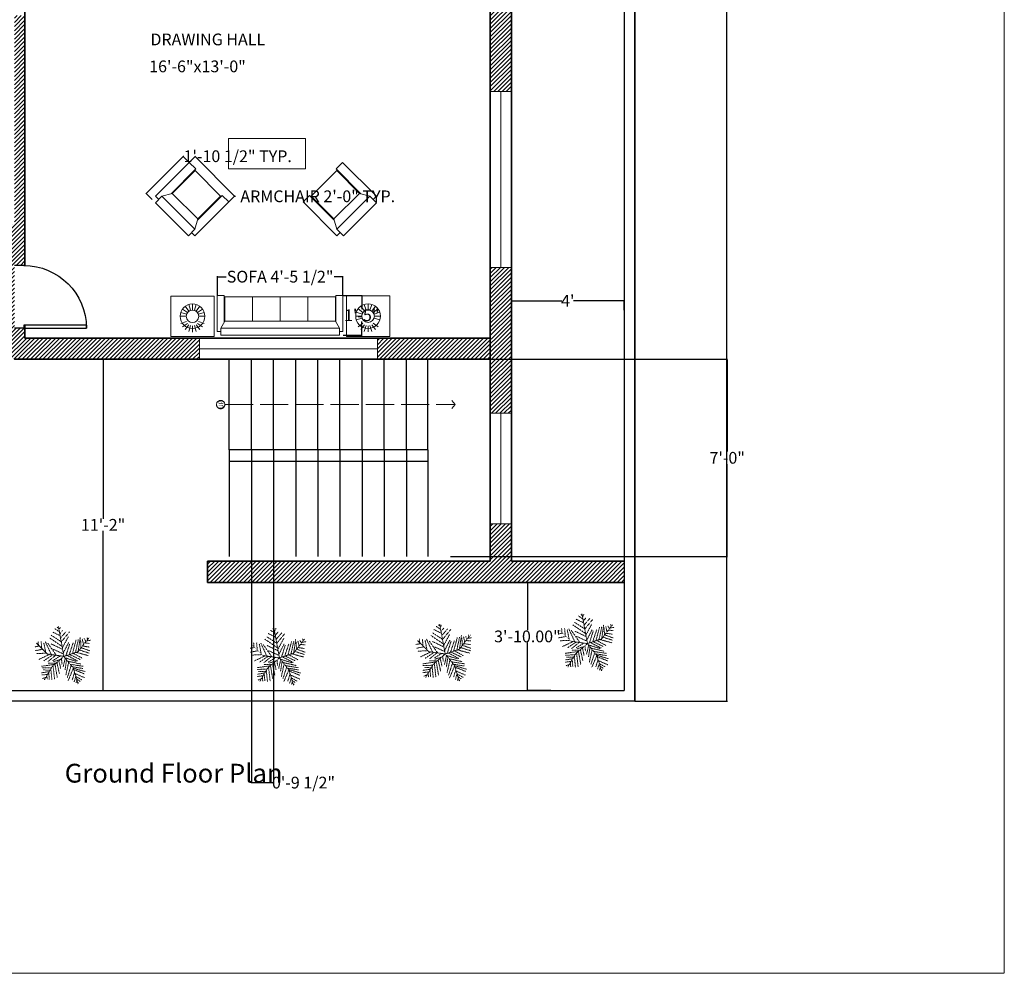
# Model space of a CAD drawing. Units: inches. Extents: x 2202345 to 2203065, y -970921 to -970107.
# Tile 2 of 5: x 2202646 to 2203065, y -970921 to -970515. Entities that reach past the tile are written whole.
import ezdxf

# ---------------------------------------------------------------- set-up
doc = ezdxf.new("R2010")
doc.units = ezdxf.units.IN
doc.header["$MEASUREMENT"] = 0
doc.linetypes.add('ACAD_ISO02W100', pattern=[15, 12, -3])
doc.linetypes.add('HIDDEN', pattern=[0.375, 0.25, -0.125])
doc.layers.get('0').update_dxf_attribs({"color": 13})
for name, color, linetype, lineweight in [('A-ANNO-DIMS', 2, 'Continuous', 18), ('A-ANNO-SYMB', 7, 'ACAD_ISO02W100', 18), ('A-ANNO-TEXT', 7, 'Continuous', 25), ('A-ANNO-TTLB', 7, 'HIDDEN', 18), ('A-AREA-IDEN', 7, 'Continuous', 18), ('A-FLOR-STRS', 252, 'Continuous', 25), ('A-WALL-PATT', 8, 'Continuous', 13), ('C-PROP', 7, 'Continuous', 25), ('doors', 252, 'Continuous', 25), ('furniture', 250, 'Continuous', 18), ('garden', 114, 'HIDDEN', 13), ('walls', 252, 'Continuous', 35), ('windows', 173, 'Continuous', 18)]:
    doc.layers.add(name, color=color, linetype=linetype, lineweight=lineweight)
doc.styles.get("Standard").update_dxf_attribs({"font": 'arial.ttf'})
doc.dimstyles.get("Standard").update_dxf_attribs({"dimtxt": 5, "dimasz": 0.18, "dimexe": 0.18, "dimexo": 0.0625, "dimgap": 0.09, "dimtad": 0, "dimtih": 1, "dimtoh": 1, "dimzin": 0, "dimdsep": 46, "dimlunit": 3, "dimtxsty": 'Standard', "dimcen": 0.09, "dimadec": 0, "dimazin": 0, "dimtfac": 1, "dimtofl": 0, "dimtmove": 0, "dimatfit": 3, "dimfxl": 1, "dimtolj": 1, "dimtzin": 0, "dimarcsym": 0})

# ---------------------------------------------------------------- blocks, each defined once
blk = doc.blocks.new('FABRIC SOFA 4S')
at = {"layer": 'furniture'}
for p, q in [((0, -51), (0, 51)), ((6, 51), (0, 51)), ((3, 54), (34, 54)), ((3, 51), (3, 54)), ((6, -51), (6, 51)), ((12, 47.63), (6, 51)), ((34, 48), (34, 54)), ((11.14, 48), (34, 48)), ((33, 23.81), (12, 23.81)), ((33, 0), (12, 0)), ((33, -23.81), (12, -23.81)), ((6, -51), (12, -47.63)), ((11.54, -48), (34, -48)), ((34, -48), (34, -54)), ((6, -51), (0, -51)), ((3, -54), (3, -51)), ((3, -54), (34, -54))]:
    blk.add_line(p, q, dxfattribs=at)
blk.add_lwpolyline([(12, -47.63), (12, 47.63), (33, 47.63), (33, -47.63)], close=True, dxfattribs=at)
blk = doc.blocks.new('FABRIC SOFA 1S')
at = {"layer": 'furniture'}
for p, q in [((0, -15.12), (0, 15.12)), ((6, 15.12), (0, 15.12)), ((3, 18.12), (34, 18.12)), ((3, 15.12), (3, 18.12)), ((6, -15.12), (6, 15.12)), ((12, 11.75), (6, 15.12)), ((34, 12.12), (34, 18.12)), ((11.33, 12.12), (34, 12.12)), ((6, -15.12), (12, -11.75)), ((11.33, -12.12), (34, -12.12)), ((34, -12.12), (34, -18.12)), ((6, -15.12), (0, -15.12)), ((3, -18.12), (3, -15.12)), ((3, -18.12), (34, -18.12))]:
    blk.add_line(p, q, dxfattribs=at)
blk.add_lwpolyline([(12, -11.75), (12, 11.75), (33, 11.75), (33, -11.75)], close=True, dxfattribs=at)
blk = doc.blocks.new('*U12')
for p, q in [((0, 0), (0, -6)), ((40, 0), (40, -6))]:
    blk.add_line(p, q)
blk.add_lwpolyline([(0, 0), (0, 40), (1.75, 40), (1.75, 0)], close=True)
blk.add_arc((0, 0), 40, 0, 90)
blk = doc.blocks.new('*D17')
at = {"layer": 'A-ANNO-DIMS', "color": 0, "lineweight": -2, "transparency": 16777216}
for p, q in [((2202675.26, -970659.11), (2202681.61, -970659.11)), ((2202681.43, -970659.29), (2202681.43, -970727.01)), ((2202681.43, -970799.93), (2202681.43, -970732.21)), ((2202681.49, -970800.11), (2202681.61, -970800.11))]:
    blk.add_line(p, q, dxfattribs=at)
at = {"layer": 'A-ANNO-DIMS', "color": 0, "transparency": 16777216}
for points in [[(2202681.4, -970659.29), (2202681.46, -970659.29), (2202681.43, -970659.11)], [(2202681.4, -970799.93), (2202681.46, -970799.93), (2202681.43, -970800.11)]]:
    blk.add_solid(points, dxfattribs=at)
at = {"layer": 'Defpoints', "color": 0, "transparency": 16777216}
for p in [(2202675.19, -970659.11), (2202681.43, -970800.11), (2202681.43, -970800.11)]:
    blk.add_point(p, dxfattribs=at)
at = {"layer": 'A-ANNO-DIMS', "color": 0, "transparency": 16777216, "insert": (2202681.43, -970729.61), "char_height": 5, "attachment_point": 5}
blk.add_mtext('\\A1;11\'-2"', dxfattribs=at)
blk = doc.blocks.new('*D18')
at = {"layer": 'A-ANNO-DIMS', "color": 0, "lineweight": -2, "transparency": 16777216}
for p, q in [((2202871.99, -970754.11), (2202861.81, -970754.11)), ((2202861.99, -970754.29), (2202861.99, -970774.46)), ((2202861.99, -970799.93), (2202861.99, -970779.75)), ((2202871.99, -970800.11), (2202861.81, -970800.11))]:
    blk.add_line(p, q, dxfattribs=at)
at = {"layer": 'A-ANNO-DIMS', "color": 0, "transparency": 16777216}
for points in [[(2202861.96, -970754.29), (2202862.02, -970754.29), (2202861.99, -970754.11)], [(2202861.96, -970799.93), (2202862.02, -970799.93), (2202861.99, -970800.11)]]:
    blk.add_solid(points, dxfattribs=at)
at = {"layer": 'Defpoints', "color": 0, "transparency": 16777216}
for p in [(2202872.05, -970754.11), (2202861.99, -970800.11), (2202872.05, -970800.11)]:
    blk.add_point(p, dxfattribs=at)
at = {"layer": 'A-ANNO-DIMS', "color": 0, "transparency": 16777216, "insert": (2202861.99, -970777.11), "char_height": 5, "attachment_point": 5}
blk.add_mtext('\\A1;3\'-10.00"', dxfattribs=at)
blk = doc.blocks.new('*D19')
at = {"layer": 'A-ANNO-DIMS', "color": 0, "lineweight": -2, "transparency": 16777216}
for p, q in [((2202855.18, -970638.23), (2202855.18, -970634)), ((2202855.36, -970634.18), (2202876.69, -970634.18)), ((2202903, -970634.18), (2202881.67, -970634.18)), ((2202903.18, -970638.23), (2202903.18, -970634))]:
    blk.add_line(p, q, dxfattribs=at)
at = {"layer": 'A-ANNO-DIMS', "color": 0, "transparency": 16777216}
for points in [[(2202855.36, -970634.15), (2202855.36, -970634.21), (2202855.18, -970634.18)], [(2202903, -970634.15), (2202903, -970634.21), (2202903.18, -970634.18)]]:
    blk.add_solid(points, dxfattribs=at)
at = {"layer": 'Defpoints', "color": 0, "transparency": 16777216}
for p in [(2202903.18, -970634.18), (2202855.18, -970638.29), (2202903.18, -970638.29)]:
    blk.add_point(p, dxfattribs=at)
at = {"layer": 'A-ANNO-DIMS', "color": 0, "transparency": 16777216, "insert": (2202879.18, -970634.18), "char_height": 5, "attachment_point": 5}
blk.add_mtext("\\A1;4'", dxfattribs=at)
blk = doc.blocks.new('*D21')
at = {"layer": 'A-ANNO-DIMS', "color": 0, "lineweight": -2, "transparency": 16777216}
for p, q in [((2202907.74, -970201.11), (2202947.11, -970201.11)), ((2202946.93, -970201.29), (2202946.93, -970500.21)), ((2202946.93, -970804.43), (2202946.93, -970505.5)), ((2202907.74, -970804.61), (2202947.11, -970804.61))]:
    blk.add_line(p, q, dxfattribs=at)
at = {"layer": 'A-ANNO-DIMS', "color": 0, "transparency": 16777216}
for points in [[(2202946.9, -970201.29), (2202946.96, -970201.29), (2202946.93, -970201.11)], [(2202946.9, -970804.43), (2202946.96, -970804.43), (2202946.93, -970804.61)]]:
    blk.add_solid(points, dxfattribs=at)
at = {"layer": 'Defpoints', "color": 0, "transparency": 16777216}
for p in [(2202907.68, -970201.11), (2202907.68, -970804.61), (2202946.93, -970804.61)]:
    blk.add_point(p, dxfattribs=at)
at = {"layer": 'A-ANNO-DIMS', "color": 0, "transparency": 16777216, "insert": (2202946.93, -970502.86), "char_height": 5, "attachment_point": 5}
blk.add_mtext("\\A1;50'", dxfattribs=at)
blk = doc.blocks.new('*U23')
for p, q in [((0, 0), (-10.5, 57)), ((-5.114, 28.097), (-24.676, 40.636)), ((-7.288, 39.707), (-21.778, 46.673)), ((-8.737, 47.138), (-17.069, 52.711)), ((-10.186, 53.64), (-13.084, 55.962)), ((-9.099, 51.782), (-6.563, 55.962)), ((-7.65, 43.423), (-2.578, 49.46)), ((-5.839, 35.992), (4.667, 48.067)), ((-5.114, 27.632), (10.463, 46.673)), ((-2.941, 16.486), (8.652, 37.85)), ((-47.498, 19.737), (-55.83, 18.344)), ((-31.5, 4.5), (-52.5, 25.5)), ((-48.585, 21.131), (-49.309, 29.026)), ((-43.513, 28.561), (-42.427, 15.558)), ((-38.442, 26.239), (-34.819, 7.663)), ((-35.544, 28.097), (-24.314, 3.947)), ((-14.533, 2.09), (-30.834, 25.31)), ((-3.665, 19.273), (-27.574, 35.527)), ((-24.314, 23.917), (-2.941, 13.7)), ((-1.129, 6.734), (9.014, 26.704)), ((3.942, 1.625), (11.187, 24.381)), ((10.101, 3.483), (17.708, 26.239)), ((16.259, 5.805), (23.142, 31.348)), ((22.055, 7.198), (27.489, 32.277)), ((27, 9), (48, 36)), ((27.127, 9.056), (31.112, 35.992)), ((31.836, 30.883), (32.561, 16.486)), ((35.096, 32.741), (37.27, 22.524)), ((36.183, 19.737), (48.137, 17.88)), ((38.719, 34.134), (41.979, 28.561)), ((40.53, 25.775), (48.862, 24.846)), ((43.791, 29.954), (51.036, 30.883)), ((44.153, 36.456), (45.239, 32.741)), ((-40.615, 13.7), (-55.105, 10.913)), ((-33.37, 6.269), (-52.207, 5.34)), ((-28.299, 3.483), (-47.86, -5.805)), ((-21.416, 3.018), (-38.079, -8.128)), ((0, 0), (-31.5, 4.5)), ((-15.982, 2.09), (-30.11, -9.521)), ((0, 0), (-22.5, -19.5)), ((-6.563, 1.161), (-21.416, -8.128)), ((-20.691, 13.7), (-1.129, 4.876)), ((0, 0), (27, 9)), ((0, 0), (18, -22.5)), ((6.478, 1.625), (26.04, -8.592)), ((11.187, 3.483), (30.749, -5.805)), ((18.07, 5.805), (35.096, -3.483)), ((24.229, 7.663), (46.688, 1.625)), ((29.662, 12.307), (48.137, 6.269)), ((33.285, 16.486), (48.862, 10.913)), ((-17.431, -15.094), (-42.789, -18.809)), ((-15.257, -12.772), (-30.11, -12.772)), ((-20.691, -18.345), (-17.793, -44.352)), ((-6.563, -5.805), (-19.967, -9.985)), ((-17.069, -15.094), (-12.721, -40.172)), ((-13.446, -11.378), (-8.737, -32.741)), ((-9.461, -8.592), (-6.201, -23.453)), ((-4.752, -3.483), (-3.665, -14.629)), ((2.493, -3.019), (-1.491, -20.202)), ((1.769, -2.555), (24.229, -9.521)), ((5.029, -6.27), (2.131, -25.775)), ((9.014, -11.378), (3.58, -35.992)), ((14.085, -16.951), (6.478, -40.172)), ((7.565, -9.056), (32.198, -14.629)), ((12.274, -15.094), (36.907, -18.809)), ((-28.299, -29.026), (-42.789, -31.348)), ((-24.314, -21.596), (-42.427, -22.06)), ((-30.834, -34.135), (-42.427, -35.528)), ((-26.849, -26.24), (-40.253, -25.775)), ((-22.5, -19.5), (-37.5, -45)), ((-32.646, -36.921), (-31.921, -44.352)), ((-29.023, -30.884), (-27.936, -43.887)), ((-25.038, -23.918), (-22.865, -45.281)), ((18.07, -22.524), (8.289, -45.745)), ((20.244, -30.419), (15.897, -44.816)), ((16.259, -19.738), (36.183, -22.989)), ((18, -22.5), (27, -52.5)), ((18.433, -22.524), (40.53, -29.026)), ((19.157, -25.311), (38.719, -33.206)), ((21.331, -32.741), (39.081, -40.636)), ((-34.457, -39.708), (-40.978, -42.494)), ((22.78, -37.85), (19.519, -48.532)), ((22.78, -38.314), (34.372, -44.816)), ((24.591, -45.745), (23.142, -50.854)), ((24.591, -43.423), (30.749, -47.603)), ((26.764, -49.925), (28.213, -50.854))]:
    blk.add_line(p, q)
blk = doc.blocks.new('STAIR-RISER')
for q in [(0, 0), (0, -84)]:
    blk.add_line((0, -38.57), q)
blk = doc.blocks.new('*D27')
at = {"layer": 'A-ANNO-DIMS', "color": 0, "lineweight": -2, "transparency": 16777216}
for p, q in [((2202718.11, -970575.26), (2202720.71, -970572.66)), ((2202720.71, -970572.91), (2202737.27, -970589.47)), ((2202734.92, -970592.07), (2202737.52, -970589.47)), ((2202737.4, -970589.59), (2202737.52, -970589.72)), ((2202737.52, -970589.72), (2202737.7, -970589.72))]:
    blk.add_line(p, q, dxfattribs=at)
at = {"layer": 'A-ANNO-DIMS', "color": 0, "transparency": 16777216}
for points in [[(2202720.73, -970572.89), (2202720.69, -970572.93), (2202720.59, -970572.78)], [(2202737.29, -970589.45), (2202737.25, -970589.49), (2202737.4, -970589.59)]]:
    blk.add_solid(points, dxfattribs=at)
at = {"layer": 'Defpoints', "color": 0, "transparency": 16777216}
for p in [(2202718.06, -970575.3), (2202737.4, -970589.59), (2202734.87, -970592.12)]:
    blk.add_point(p, dxfattribs=at)
at = {"layer": 'A-ANNO-DIMS', "color": 0, "transparency": 16777216, "insert": (2202772.77, -970589.72), "char_height": 5, "attachment_point": 5}
blk.add_mtext('\\A1;ARMCHAIR 2\'-0" TYP.', dxfattribs=at)
blk = doc.blocks.new('*D28')
at = {"layer": 'A-ANNO-DIMS', "color": 0, "lineweight": -2, "transparency": 16777216}
for p, q in [((2202699.9, -970588.42), (2202715.41, -970572.91)), ((2202718.02, -970575.26), (2202715.41, -970572.66)), ((2202715.54, -970572.78), (2202715.67, -970572.66)), ((2202715.67, -970572.66), (2202715.85, -970572.66)), ((2202702.25, -970591.03), (2202699.65, -970588.42))]:
    blk.add_line(p, q, dxfattribs=at)
at = {"layer": 'A-ANNO-DIMS', "color": 0, "transparency": 16777216}
for points in [[(2202715.39, -970572.89), (2202715.44, -970572.93), (2202715.54, -970572.78)], [(2202699.88, -970588.4), (2202699.92, -970588.44), (2202699.77, -970588.55)]]:
    blk.add_solid(points, dxfattribs=at)
at = {"layer": 'Defpoints', "color": 0, "transparency": 16777216}
for p in [(2202715.54, -970572.78), (2202718.06, -970575.3), (2202702.3, -970591.07)]:
    blk.add_point(p, dxfattribs=at)
at = {"layer": 'A-ANNO-DIMS', "color": 0, "transparency": 16777216, "insert": (2202738.71, -970572.66), "char_height": 5, "attachment_point": 5}
blk.add_mtext('\\A1;1\'-10 1/2" TYP.', dxfattribs=at)
blk = doc.blocks.new('*D29')
at = {"layer": 'A-ANNO-DIMS', "color": 0, "lineweight": -2, "transparency": 16777216}
for p, q in [((2202730.04, -970631.9), (2202730.04, -970623.76)), ((2202730.22, -970623.94), (2202733.73, -970623.94)), ((2202783.31, -970623.94), (2202779.79, -970623.94)), ((2202783.49, -970631.9), (2202783.49, -970623.76))]:
    blk.add_line(p, q, dxfattribs=at)
at = {"layer": 'A-ANNO-DIMS', "color": 0, "transparency": 16777216}
for points in [[(2202730.22, -970623.91), (2202730.22, -970623.97), (2202730.04, -970623.94)], [(2202783.31, -970623.91), (2202783.31, -970623.97), (2202783.49, -970623.94)]]:
    blk.add_solid(points, dxfattribs=at)
at = {"layer": 'Defpoints', "color": 0, "transparency": 16777216}
for p in [(2202730.04, -970623.94), (2202730.04, -970631.96), (2202783.49, -970631.96)]:
    blk.add_point(p, dxfattribs=at)
at = {"layer": 'A-ANNO-DIMS', "color": 0, "transparency": 16777216, "insert": (2202756.76, -970623.94), "char_height": 5, "attachment_point": 5}
blk.add_mtext('\\A1;SOFA 4\'-5 1/2"', dxfattribs=at)
blk = doc.blocks.new('*D30')
at = {"layer": 'A-ANNO-DIMS', "color": 0, "lineweight": -2, "transparency": 16777216}
for p, q in [((2202783.55, -970631.96), (2202791.68, -970631.96)), ((2202791.5, -970632.14), (2202791.5, -970637.73)), ((2202791.5, -970648.61), (2202791.5, -970643.02)), ((2202783.55, -970648.79), (2202791.68, -970648.79))]:
    blk.add_line(p, q, dxfattribs=at)
at = {"layer": 'A-ANNO-DIMS', "color": 0, "transparency": 16777216}
for points in [[(2202791.47, -970632.14), (2202791.53, -970632.14), (2202791.5, -970631.96)], [(2202791.47, -970648.61), (2202791.53, -970648.61), (2202791.5, -970648.79)]]:
    blk.add_solid(points, dxfattribs=at)
at = {"layer": 'Defpoints', "color": 0, "transparency": 16777216}
for p in [(2202783.49, -970631.96), (2202791.5, -970631.96), (2202783.49, -970648.79)]:
    blk.add_point(p, dxfattribs=at)
at = {"layer": 'A-ANNO-DIMS', "color": 0, "transparency": 16777216, "insert": (2202791.5, -970640.37), "char_height": 5, "attachment_point": 5}
blk.add_mtext('\\A1;1\'-5"', dxfattribs=at)
blk = doc.blocks.new('*D41')
at = {"layer": 'A-ANNO-DIMS', "color": 0, "lineweight": -2, "transparency": 16777216}
for p, q in [((2202744.54, -970743.17), (2202744.54, -970839.54)), ((2202753.96, -970743.17), (2202753.96, -970839.54)), ((2202744.72, -970839.36), (2202753.78, -970839.36)), ((2202753.96, -970839.36), (2202754.14, -970839.36))]:
    blk.add_line(p, q, dxfattribs=at)
at = {"layer": 'A-ANNO-DIMS', "color": 0, "transparency": 16777216}
for points in [[(2202744.72, -970839.33), (2202744.72, -970839.39), (2202744.54, -970839.36)], [(2202753.78, -970839.33), (2202753.78, -970839.39), (2202753.96, -970839.36)]]:
    blk.add_solid(points, dxfattribs=at)
at = {"layer": 'Defpoints', "color": 0, "transparency": 16777216}
for p in [(2202744.54, -970743.11), (2202753.96, -970743.11), (2202753.96, -970839.36)]:
    blk.add_point(p, dxfattribs=at)
at = {"layer": 'A-ANNO-DIMS', "color": 0, "transparency": 16777216, "insert": (2202766.7, -970839.36), "char_height": 5, "attachment_point": 5}
blk.add_mtext('\\A1;0\'-9 1/2"', dxfattribs=at)
blk = doc.blocks.new('*D42')
at = {"layer": 'A-ANNO-DIMS', "color": 0, "lineweight": -2, "transparency": 16777216}
for p, q in [((2202819.67, -970659.11), (2202947.21, -970659.11)), ((2202947.03, -970659.29), (2202947.03, -970698.42)), ((2202947.03, -970742.84), (2202947.03, -970703.71)), ((2202829.33, -970743.02), (2202947.21, -970743.02))]:
    blk.add_line(p, q, dxfattribs=at)
at = {"layer": 'A-ANNO-DIMS', "color": 0, "transparency": 16777216}
for points in [[(2202947, -970659.29), (2202947.06, -970659.29), (2202947.03, -970659.11)], [(2202947, -970742.84), (2202947.06, -970742.84), (2202947.03, -970743.02)]]:
    blk.add_solid(points, dxfattribs=at)
at = {"layer": 'Defpoints', "color": 0, "transparency": 16777216}
for p in [(2202819.6, -970659.11), (2202947.03, -970659.11), (2202829.26, -970743.02)]:
    blk.add_point(p, dxfattribs=at)
at = {"layer": 'A-ANNO-DIMS', "color": 0, "transparency": 16777216, "insert": (2202947.03, -970701.06), "char_height": 5, "attachment_point": 5}
blk.add_mtext('\\A1;7\'-0"', dxfattribs=at)

msp = doc.modelspace()

# ---------------------------------------------------------------- hatches: boundary and pattern name
at = {"layer": 'A-WALL-PATT'}
h = msp.add_hatch(dxfattribs=at)
h.set_pattern_fill('ANSI31', color=256, scale=10)
h.set_pattern_definition([(45, (0, 0), (-0.8838834765, 0.8838834765), [])])
h.paths.add_polyline_path([(2202648.182, -970512.768), (2202644.707, -970512.768, -0.0110733), (2202643.682, -970512.746), (2202643.682, -970601.606), (2202609.913, -970601.606), (2202609.913, -970610.606), (2202643.682, -970610.606), (2202643.682, -970619.168), (2202647.677, -970619.168, -0.0047326), (2202648.182, -970619.173)])
h.paths.add_polyline_path([(2202643.682, -970610.606), (2202636.037, -970610.606), (2202636.037, -970659.106), (2202643.682, -970659.106)])
h.paths.add_polyline_path([(2202722.39, -970654.606), (2202722.39, -970650.106), (2202648.182, -970650.106), (2202648.182, -970645.806), (2202647.677, -970645.806), (2202643.682, -970645.806), (2202643.682, -970659.106), (2202722.39, -970659.106)])
h.paths.add_polyline_path([(2202846.182, -970650.106), (2202798.148, -970650.106), (2202798.148, -970659.106), (2202846.182, -970659.106)])
h.paths.add_polyline_path([(2202855.182, -970619.995), (2202846.182, -970619.995), (2202846.182, -970682.124), (2202855.182, -970682.124)])
h.paths.add_polyline_path([(2202855.182, -970434.646), (2202846.182, -970434.646), (2202846.182, -970545.038), (2202855.182, -970545.038)])
h.paths.add_polyline_path([(2202903.182, -970745.106), (2202855.182, -970745.106), (2202855.182, -970729.208), (2202846.182, -970729.208), (2202846.182, -970745.106), (2202725.91, -970745.106), (2202725.91, -970754.106), (2202903.182, -970754.106)])
h.paths.add_polyline_path([(2202846.182, -970489.606), (2202767.486, -970489.606, -0.1570508), (2202766.685, -970489.864), (2202739.229, -970489.864, -0.1570508), (2202738.428, -970489.606), (2202685.343, -970489.606), (2202685.343, -970494.106), (2202846.182, -970494.106)])
h.paths.add_polyline_path([(2202648.182, -970477.106), (2202594.182, -970477.106), (2202594.182, -970352.606), (2202624.243, -970352.606), (2202624.243, -970348.106), (2202575.482, -970348.106), (2202575.482, -970352.606), (2202589.682, -970352.606), (2202589.682, -970412.606), (2202505.682, -970412.606), (2202505.682, -970417.106), (2202589.682, -970417.106), (2202589.682, -970477.106), (2202580.925, -970477.106), (2202580.925, -970481.606), (2202643.682, -970481.606), (2202643.682, -970489.606), (2202644.707, -970489.606), (2202648.182, -970489.606)])
h.paths.add_polyline_path([(2202505.682, -970305.515), (2202496.682, -970305.515), (2202496.682, -970378.877), (2202501.298, -970378.877), (2202505.682, -970378.877)])
h.paths.add_polyline_path([(2202540.998, -970348.106), (2202505.682, -970348.106), (2202505.682, -970352.606), (2202540.998, -970352.606)], flags=17)
h.paths.add_polyline_path([(2202505.682, -970452.918), (2202496.682, -970452.918), (2202496.682, -970516.267), (2202505.682, -970516.267)])
h.paths.add_polyline_path([(2202505.682, -970210.106), (2202898.682, -970210.106), (2202898.682, -970294.106), (2202889.459, -970294.106), (2202889.459, -970303.106), (2202907.682, -970303.106), (2202907.682, -970201.106), (2202496.682, -970201.106), (2202496.682, -970242.728), (2202505.682, -970242.728)])
h.paths.add_polyline_path([(2202678.182, -970210.106), (2202673.682, -970210.106), (2202673.682, -970348.106), (2202664.243, -970348.106), (2202664.243, -970352.606), (2202686.569, -970352.606), (2202686.569, -970348.106), (2202678.182, -970348.106)])
h.paths.add_polyline_path([(2202752.572, -970321.843), (2202794.204, -970321.843), (2202794.204, -970314.185), (2202752.572, -970314.185)], flags=9)
h.paths.add_polyline_path([(2202750.562, -970312.127), (2202793.125, -970312.127), (2202793.125, -970304.366), (2202750.562, -970304.366)], flags=9)

# ---------------------------------------------------------------- linework, layer by layer
at = {"layer": 'A-ANNO-SYMB'}
for p, q in [((2202831.222, -970678.392), (2202829.868, -970676.607)), ((2202733.223, -970678.392), (2202831.222, -970678.392)), ((2202829.868, -970680.02), (2202831.222, -970678.392))]:
    msp.add_line(p, q, dxfattribs=at)
msp.add_circle((2202731.453, -970678.392), 1.77, dxfattribs=at)
at = {"layer": 'A-ANNO-TTLB'}
for p, q in [((2203064.943, -970920.555), (2203064.943, -970106.63)), ((2202344.52, -970920.555), (2203064.943, -970920.555))]:
    msp.add_line(p, q, dxfattribs=at)
at = {"layer": 'A-FLOR-STRS'}
for p, q in [((2202819.605, -970697.679), (2202735.117, -970697.679)), ((2202819.605, -970702.679), (2202735.117, -970702.679))]:
    msp.add_line(p, q, dxfattribs=at)
at = {"layer": 'C-PROP'}
for p, q in [((2202903.182, -970303.106), (2202903.182, -970800.106)), ((2202459.682, -970800.106), (2202903.182, -970800.106)), ((2202459.682, -970804.606), (2202907.682, -970804.606))]:
    msp.add_line(p, q, dxfattribs=at)
at = {"layer": 'furniture'}
for p, q in [((2202734.837, -970578.005), (2202734.837, -970565.145)), ((2202734.837, -970565.145), (2202767.568, -970565.145)), ((2202767.568, -970565.145), (2202767.568, -970578.005)), ((2202767.568, -970578.005), (2202734.837, -970578.005)), ((2202717.843, -970635.807), (2202718.641, -970638.264)), ((2202719.463, -970635.551), (2202719.463, -970638.134)), ((2202721.083, -970635.807), (2202720.284, -970638.264)), ((2202792.552, -970635.732), (2202793.354, -970638.202)), ((2202794.181, -970635.474), (2202794.181, -970638.071)), ((2202795.81, -970635.732), (2202795.007, -970638.202)), ((2202714.477, -970639.173), (2202716.934, -970639.972)), ((2202715.221, -970637.712), (2202717.311, -970639.23)), ((2202716.381, -970636.552), (2202717.9, -970638.642)), ((2202722.544, -970636.552), (2202721.026, -970638.642)), ((2202723.704, -970637.712), (2202721.614, -970639.23)), ((2202724.448, -970639.173), (2202721.992, -970639.972)), ((2202789.167, -970639.116), (2202791.638, -970639.919)), ((2202789.916, -970637.647), (2202792.017, -970639.174)), ((2202791.082, -970636.481), (2202792.609, -970638.582)), ((2202797.28, -970636.481), (2202795.753, -970638.582)), ((2202798.446, -970637.647), (2202796.344, -970639.174)), ((2202799.195, -970639.116), (2202796.724, -970639.919)), ((2202714.22, -970640.793), (2202716.803, -970640.793)), ((2202714.477, -970643.878), (2202716.934, -970643.08)), ((2202715.221, -970645.34), (2202717.311, -970643.821)), ((2202716.381, -970646.499), (2202717.9, -970644.409)), ((2202722.544, -970646.499), (2202721.026, -970644.409)), ((2202723.704, -970645.34), (2202721.614, -970643.821)), ((2202724.448, -970643.878), (2202721.992, -970643.08)), ((2202724.705, -970640.793), (2202722.122, -970640.793)), ((2202788.909, -970640.746), (2202791.507, -970640.746)), ((2202789.167, -970642.375), (2202791.638, -970641.572)), ((2202789.916, -970645.309), (2202792.017, -970643.782)), ((2202791.082, -970646.475), (2202792.609, -970644.374)), ((2202797.28, -970646.475), (2202795.753, -970644.374)), ((2202798.446, -970645.309), (2202796.344, -970643.782)), ((2202799.195, -970642.375), (2202796.724, -970641.572)), ((2202799.453, -970640.746), (2202796.855, -970640.746)), ((2202717.843, -970647.244), (2202718.641, -970644.787)), ((2202719.463, -970647.501), (2202719.463, -970644.917)), ((2202721.083, -970647.244), (2202720.284, -970644.787)), ((2202792.552, -970647.224), (2202793.354, -970644.753)), ((2202794.181, -970647.482), (2202794.181, -970644.884)), ((2202795.81, -970647.224), (2202795.007, -970644.753))]:
    msp.add_line(p, q, dxfattribs=at)
for points in [[(2202728.624, -970649.357), (2202728.624, -970632.23), (2202710.301, -970632.23), (2202710.301, -970649.357)], [(2202803.393, -970649.357), (2202803.393, -970632.134), (2202784.969, -970632.134), (2202784.969, -970649.357)]]:
    msp.add_lwpolyline(points, close=True, dxfattribs=at)
for centre, radius in [((2202719.463, -970640.793), 5.243), ((2202794.181, -970640.746), 5.272), ((2202719.463, -970640.793), 2.659), ((2202794.181, -970640.746), 2.674)]:
    msp.add_circle(centre, radius, dxfattribs=at)
at = {"layer": 'walls'}
for p, q in [((2202907.682, -970201.106), (2202907.682, -970804.606)), ((2202855.182, -970303.106), (2202855.182, -970745.106)), ((2202846.182, -970378.414), (2202846.182, -970745.106)), ((2202648.182, -970477.106), (2202648.182, -970619.173)), ((2202648.182, -970644.641), (2202648.182, -970650.106)), ((2202648.182, -970650.106), (2202846.182, -970650.106)), ((2202643.682, -970659.106), (2202846.182, -970659.106)), ((2202725.91, -970745.106), (2202846.182, -970745.106)), ((2202725.91, -970745.106), (2202725.91, -970754.106)), ((2202855.182, -970745.106), (2202903.182, -970745.106)), ((2202725.91, -970754.106), (2202903.182, -970754.106))]:
    msp.add_line(p, q, dxfattribs=at)
at = {"layer": 'windows'}
for p, q in [((2202846.182, -970545.038), (2202855.182, -970545.038)), ((2202855.182, -970545.038), (2202850.682, -970545.038)), ((2202850.682, -970545.038), (2202850.682, -970619.995)), ((2202850.682, -970619.995), (2202846.182, -970619.995)), ((2202846.182, -970619.995), (2202855.182, -970619.995)), ((2202722.39, -970650.106), (2202722.39, -970659.106)), ((2202798.148, -970654.606), (2202798.148, -970650.106)), ((2202798.148, -970650.106), (2202798.148, -970659.106)), ((2202722.39, -970659.106), (2202722.39, -970654.606)), ((2202722.39, -970654.606), (2202798.148, -970654.606)), ((2202846.182, -970682.124), (2202855.182, -970682.124)), ((2202855.182, -970682.124), (2202850.682, -970682.124)), ((2202850.682, -970682.124), (2202850.682, -970729.208)), ((2202850.682, -970729.208), (2202846.182, -970729.208)), ((2202846.182, -970729.208), (2202855.182, -970729.208))]:
    msp.add_line(p, q, dxfattribs=at)

# ---------------------------------------------------------------- block references
at = {"layer": 'A-FLOR-STRS'}
for p in [(2202735.117, -970659.106), (2202744.538, -970659.106), (2202753.959, -970659.106), (2202763.38, -970659.106), (2202772.801, -970659.106), (2202782.222, -970659.106), (2202791.643, -970659.106), (2202801.064, -970659.106), (2202810.485, -970659.106), (2202819.605, -970659.106)]:
    msp.add_blockref('STAIR-RISER', p, dxfattribs=at)
at = {"layer": 'doors', "xscale": -0.6659591083613691, "yscale": 0.6659591083613691, "zscale": 0.6659591083613691, "rotation": 270}
msp.add_blockref('*U12', (2202647.677, -970645.806), dxfattribs=at)
at = {"layer": 'furniture'}
for name, p, xscale, yscale, zscale, rotation in [('FABRIC SOFA 1S', (2202710.702, -970599.478), -0.6558392697258925, 0.6558392697258923, 0.6558392697258923, 225.0000000000571), ('FABRIC SOFA 1S', (2202790.693, -970599.478), 0.6558392697258925, 0.6558392697258925, 0.6558392697258925, 134.9999999999428), ('FABRIC SOFA 4S', (2202756.762, -970648.788), 0.4948907828209233, 0.4948907828209233, 0.4948907828209233, 89.99999999999991)]:
    msp.add_blockref(name, p, dxfattribs=dict(at, xscale=xscale, yscale=yscale, zscale=zscale, rotation=rotation))
at = {"layer": 'garden', "xscale": 0.2228486455557245, "yscale": 0.2228486455557245, "zscale": 0.2228486455557245}
for p in [(2202887.537, -970780.159), (2202664.758, -970785.628), (2202756.469, -970786.249), (2202827.016, -970784.593)]:
    msp.add_blockref('*U23', p, dxfattribs=at)

# ---------------------------------------------------------------- texts
at = {"layer": 'A-ANNO-SYMB'}
msp.add_text('UP', height=2, rotation=90, dxfattribs=at).set_placement((2202732.593, -970680.229))
at = {"layer": 'A-ANNO-TEXT'}
msp.add_text('Ground Floor Plan', height=8, dxfattribs=at).set_placement((2202665.093, -970839.345))
at = {"layer": 'A-AREA-IDEN'}
for s, p in [('DRAWING HALL', (2202701.559, -970525.431)), ('16\'-6"x13\'-0"', (2202701.047, -970536.903))]:
    msp.add_text(s, height=5, dxfattribs=at).set_placement(p)

# ---------------------------------------------------------------- dimensions: what is measured, and where the dimension line sits
at = {"layer": 'A-ANNO-DIMS'}
for base, p1, p2, angle, text, override, picture, middle in [((2202946.927, -970804.606), (2202907.682, -970201.106), (2202907.682, -970804.606), 90, "50'", {"dimclrd": 0, "dimclre": 0, "dimclrt": 0}, '*D21', (2202946.927, -970502.856)), ((2202715.542, -970572.783), (2202702.296, -970591.072), (2202718.064, -970575.305), 45, '<> TYP.', {"dimdec": 1, "dimlfac": 1, "dimrnd": 0, "dimzin": 1, "dimdsep": 46, "dimlunit": 4, "dimfrac": 2}, '*D28', (2202738.71, -970572.656)), ((2202737.396, -970589.594), (2202718.064, -970575.305), (2202734.874, -970592.116), 315, 'ARMCHAIR <> TYP.', {"dimdec": 1, "dimlfac": 1, "dimrnd": 0, "dimzin": 1, "dimdsep": 46, "dimlunit": 4, "dimfrac": 2}, '*D27', (2202772.775, -970589.722)), ((2202730.038, -970623.945), (2202783.486, -970631.962), (2202730.038, -970631.962), 180, 'SOFA <>', {"dimdec": 1, "dimlfac": 1, "dimrnd": 0, "dimzin": 1, "dimdsep": 46, "dimlunit": 4, "dimfrac": 2}, '*D29', (2202756.762, -970623.945)), ((2202681.432, -970800.106), (2202675.194, -970659.106), (2202681.432, -970800.106), 90, '11\'-2"', {"dimclrd": 0, "dimclre": 0, "dimclrt": 0}, '*D17', (2202681.432, -970729.606))]:
    dim = msp.add_linear_dim(base=base, p1=p1, p2=p2, angle=angle, text=text, dimstyle='Standard', override=override, dxfattribs=at)
    dim.commit()
    dim.dimension.update_dxf_attribs({"geometry": picture, "text_midpoint": middle})
for base, p1, p2, override, picture, middle in [((2202903.182, -970634.177), (2202855.182, -970638.289), (2202903.182, -970638.289), {"dimclrd": 0, "dimclre": 0, "dimclrt": 0}, '*D19', (2202879.182, -970634.177)), ((2202753.959, -970839.356), (2202744.538, -970743.106), (2202753.959, -970743.106), {"dimdec": 1, "dimlfac": 1, "dimrnd": 0, "dimzin": 1, "dimdsep": 46, "dimlunit": 4, "dimfrac": 2}, '*D41', (2202766.7, -970839.356))]:
    dim = msp.add_linear_dim(base=base, p1=p1, p2=p2, dimstyle='Standard', override=override, dxfattribs=at)
    dim.commit()
    dim.dimension.update_dxf_attribs({"geometry": picture, "text_midpoint": middle})
for base, p1, p2, override, picture, middle in [((2202791.503, -970631.962), (2202783.486, -970648.788), (2202783.486, -970631.962), {"dimdec": 1, "dimlfac": 1, "dimrnd": 0, "dimzin": 1, "dimdsep": 46, "dimlunit": 4, "dimfrac": 2}, '*D30', (2202791.503, -970640.375)), ((2202947.029, -970659.106), (2202829.264, -970743.021), (2202819.605, -970659.106), {"dimdec": 1, "dimlfac": 1, "dimrnd": 0, "dimzin": 1, "dimdsep": 46, "dimlunit": 4, "dimfrac": 2}, '*D42', (2202947.029, -970701.063)), ((2202861.99, -970800.106), (2202872.055, -970754.106), (2202872.055, -970800.106), {"dimclrd": 0, "dimclre": 0, "dimclrt": 0}, '*D18', (2202861.99, -970777.106))]:
    dim = msp.add_linear_dim(base=base, p1=p1, p2=p2, angle=90, dimstyle='Standard', override=override, dxfattribs=at)
    dim.commit()
    dim.dimension.update_dxf_attribs({"geometry": picture, "text_midpoint": middle})

doc.saveas('drawing.dxf')
